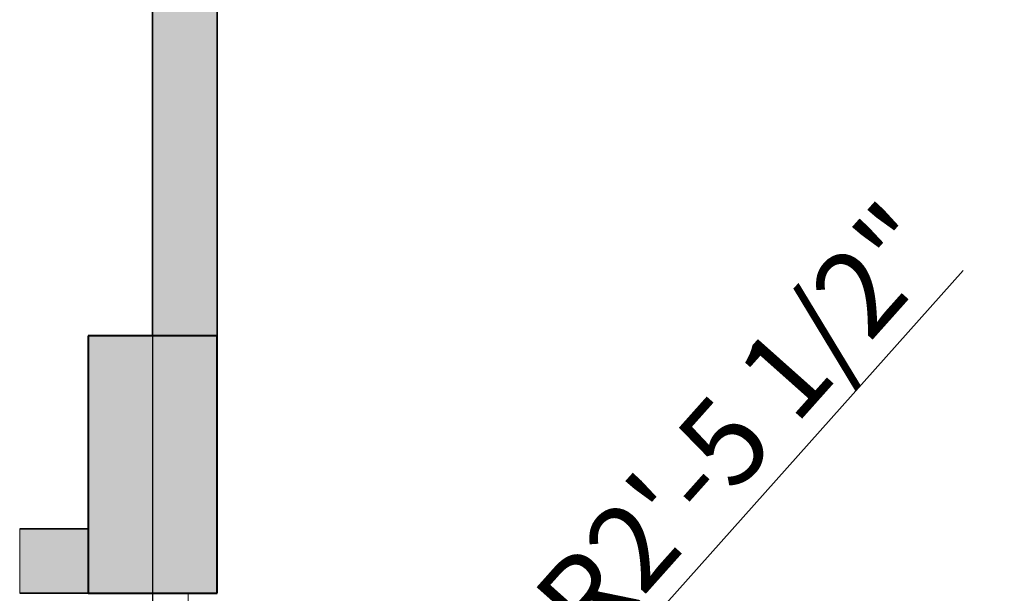
# Model space of a CAD drawing. Units: inches. Extents: x 2656 to 9931, y 1941 to 3068.
# Tile 14 of 46: x 2863 to 2932, y 2426 to 2466. Entities that reach past the tile are written whole.
import ezdxf

# ---------------------------------------------------------------- set-up
doc = ezdxf.new("R2010")
doc.units = ezdxf.units.IN
for name, color, linetype, lineweight in [('A-ANNO-DIMS', 2, 'Continuous', 18), ('A-COLS', 7, 'Continuous', 40), ('A-COLS-PATT', 146, 'Continuous', 13), ('A-DOOR', 3, 'Continuous', 18), ('A-WALL', 7, 'Continuous', 35), ('A-WALL-PATT', 251, 'Continuous', 13)]:
    doc.layers.add(name, color=color, linetype=linetype, lineweight=lineweight)
doc.styles.get("Standard").update_dxf_attribs({"font": 'arial.ttf'})
doc.dimstyles.new('ISO-25', dxfattribs={"dimtxt": 6, "dimasz": 2.5, "dimexe": 1.25, "dimexo": 0.625, "dimtad": 1, "dimdec": 0, "dimlunit": 3, "dimtxsty": 'Standard', "dimcen": 2.5, "dimadec": 0, "dimazin": 0, "dimtfac": 1, "dimtdec": 0, "dimtmove": 0, "dimatfit": 3, "dimfxl": 1, "dimarcsym": 0})

# ---------------------------------------------------------------- blocks, each defined once
blk = doc.blocks.new('DOOR-BEDROOM-HALL')
for p, q in [((-0.043, 0), (-0.043, 36)), ((2.43, 36), (2.43, 34)), ((38.43, 3), (2.43, 3)), ((2.43, 3), (2.43, 2)), ((38.43, 2), (38.43, 3)), ((2.43, 0), (2.43, 2)), ((2.43, 2), (38.43, 2))]:
    blk.add_line(p, q)
blk.add_arc((9.014, 5.243), 29.501, 353.68892, 102.89617)
blk = doc.blocks.new('*D102')
at = {"layer": 'A-ANNO-DIMS', "color": 0, "lineweight": -2, "transparency": 16777216}
for p, q in [((2998.157, 2604.975), (2998.157, 2009.273)), ((2872.157, 2564.712), (2872.157, 2009.273)), ((2874.657, 2010.523), (2995.657, 2010.523))]:
    blk.add_line(p, q, dxfattribs=at)
at = {"layer": 'A-ANNO-DIMS', "color": 0, "transparency": 16777216}
for points in [[(2874.657, 2010.939), (2874.657, 2010.106), (2872.157, 2010.523)], [(2995.657, 2010.939), (2995.657, 2010.106), (2998.157, 2010.523)]]:
    blk.add_solid(points, dxfattribs=at)
at = {"layer": 'Defpoints', "color": 0, "transparency": 16777216}
for p in [(2998.157, 2605.6), (2872.157, 2565.337), (2998.157, 2010.523)]:
    blk.add_point(p, dxfattribs=at)
at = {"layer": 'A-ANNO-DIMS', "color": 0, "transparency": 16777216, "insert": (2935.157, 2014.211), "char_height": 6, "attachment_point": 5}
blk.add_mtext('10\'-6"', dxfattribs=at)
blk = doc.blocks.new('*D185')
at = {"layer": 'A-ANNO-DIMS', "color": 0, "lineweight": -2, "transparency": 16777216}
for p, q in [((2928.735, 2448.665), (2902.506, 2419.234)), ((2881.214, 2395.343), (2900.842, 2417.367))]:
    blk.add_line(p, q, dxfattribs=at)
at = {"layer": 'A-ANNO-DIMS', "color": 0, "transparency": 16777216}
blk.add_solid([(2902.195, 2419.511), (2902.817, 2418.957), (2900.842, 2417.367)], dxfattribs=at)
at = {"layer": 'Defpoints', "color": 0, "transparency": 16777216}
for p in [(2900.842, 2417.367), (2881.214, 2395.343)]:
    blk.add_point(p, dxfattribs=at)
at = {"layer": 'A-ANNO-DIMS', "color": 0, "transparency": 16777216, "insert": (2913.669, 2437.362), "char_height": 6, "attachment_point": 5, "rotation": 48.29259}
blk.add_mtext('R2\'-5 1/2"', dxfattribs=at)

msp = doc.modelspace()

# ---------------------------------------------------------------- hatches: boundary and pattern name
at = {"layer": 'A-COLS-PATT'}
h = msp.add_hatch(color=256, dxfattribs=at)
h.dxf.hatch_style = 1
h.paths.add_polyline_path([(2752.157, 2623.6), (2743.157, 2623.6), (2743.157, 2605.6), (2752.157, 2605.6)])
h.paths.add_polyline_path([(2876.657, 2623.6), (2858.657, 2623.6), (2858.657, 2614.6), (2876.657, 2614.6)])
h.paths.add_polyline_path([(2998.157, 2623.6), (2989.157, 2623.6), (2989.157, 2614.6), (2989.157, 2605.6), (2998.157, 2605.6)])
h.paths.add_polyline_path([(2998.157, 2444.1), (2989.157, 2444.1), (2989.157, 2426.1), (2998.157, 2426.1)])
h.paths.add_polyline_path([(2876.657, 2444.1), (2867.657, 2444.1), (2867.657, 2426.1), (2876.657, 2426.1)])
h.paths.add_polyline_path([(2752.157, 2444.1), (2743.157, 2444.1), (2743.157, 2426.1), (2752.157, 2426.1)])
h.paths.add_polyline_path([(2752.157, 2300.1), (2743.157, 2300.1), (2743.157, 2282.1), (2752.157, 2282.1)])
h.paths.add_polyline_path([(2876.657, 2300.1), (2867.657, 2300.1), (2867.657, 2282.1), (2876.657, 2282.1)])
h.paths.add_polyline_path([(2998.157, 2300.1), (2989.157, 2300.1), (2989.157, 2282.1), (2998.157, 2282.1)])
h.paths.add_polyline_path([(2998.157, 2184.6), (2989.157, 2184.6), (2989.157, 2166.6), (2998.157, 2166.6)])
h.paths.add_polyline_path([(2876.657, 2175.6), (2858.657, 2175.6), (2858.657, 2166.6), (2876.657, 2166.6)])
h.paths.add_polyline_path([(2752.157, 2184.6), (2743.157, 2184.6), (2743.157, 2166.6), (2752.157, 2166.6)])
at = {"layer": 'A-WALL-PATT'}
h = msp.add_hatch(color=256, dxfattribs=at)
h.dxf.hatch_style = 1
h.paths.add_polyline_path([(2858.657, 2623.6), (2752.157, 2623.6), (2752.157, 2614.6), (2858.657, 2614.6)])
h.paths.add_polyline_path([(2893.087, 2623.6), (2876.657, 2623.6), (2876.657, 2614.6), (2893.087, 2614.6), (2893.087, 2619.1)])
h.paths.add_polyline_path([(2946.514, 2623.6), (2917.087, 2623.6), (2917.087, 2614.6), (2946.514, 2614.6), (2946.514, 2619.1)])
h.paths.add_polyline_path([(2989.157, 2623.6), (2970.514, 2623.6), (2970.514, 2614.6), (2989.157, 2614.6)])
h.paths.add_polyline_path([(2998.157, 2605.6), (2989.157, 2605.6), (2989.157, 2523.881), (2998.157, 2523.881)])
h.paths.add_polyline_path([(2935.157, 2614.6), (2930.657, 2614.6), (2930.657, 2554.6), (2876.657, 2554.6), (2876.657, 2565.337), (2872.157, 2565.337), (2872.157, 2444.1), (2876.657, 2444.1), (2876.657, 2550.1), (2946.472, 2550.1), (2946.472, 2554.6), (2935.157, 2554.6)])
h.paths.add_polyline_path([(2989.157, 2554.6), (2982.11, 2554.6), (2976.574, 2554.6), (2976.574, 2550.1), (2982.11, 2550.1), (2989.157, 2550.1)])
h.paths.add_polyline_path([(2876.657, 2614.6), (2872.157, 2614.6), (2872.157, 2595.003), (2876.657, 2595.003)], flags=0)
h.paths.add_polyline_path([(2752.157, 2605.6), (2743.157, 2605.6), (2743.157, 2544.033), (2752.157, 2544.033)])
h.paths.add_polyline_path([(2752.157, 2426.1), (2743.157, 2426.1), (2743.157, 2300.1), (2752.157, 2300.1)])
h.paths.add_polyline_path([(2821.134, 2430.6), (2752.157, 2430.6), (2752.157, 2426.1), (2821.134, 2426.1)])
h.paths.add_polyline_path([(2867.657, 2430.6), (2862.876, 2430.6), (2862.876, 2426.1), (2867.657, 2426.1)])
h.paths.add_polyline_path([(2752.157, 2484.033), (2747.657, 2484.033), (2743.157, 2484.033), (2743.157, 2444.1), (2752.157, 2444.1)])
h.paths.add_polyline_path([(2998.157, 2426.1), (2989.157, 2426.1), (2989.157, 2390.1), (2872.157, 2390.1), (2872.157, 2385.6), (2876.657, 2385.6), (2989.157, 2385.6), (2989.157, 2365.037), (2998.157, 2365.037)])
h.paths.add_polyline_path([(2998.157, 2463.881), (2993.657, 2463.881), (2989.157, 2463.881), (2989.157, 2444.1), (2998.157, 2444.1)])
h.paths.add_polyline_path([(2998.157, 2319.88), (2989.157, 2319.88), (2989.157, 2300.1), (2998.157, 2300.1)])
h.paths.add_polyline_path([(2998.157, 2282.1), (2989.157, 2282.1), (2989.157, 2253.6), (2982.058, 2253.6), (2982.058, 2249.1), (2989.157, 2249.1), (2998.157, 2249.1)])
h.paths.add_polyline_path([(2931.542, 2253.6), (2923.796, 2253.6), (2923.796, 2249.1), (2931.542, 2249.1)])
h.paths.add_polyline_path([(2876.657, 2282.1), (2872.157, 2282.1), (2872.157, 2184.6), (2872.157, 2175.6), (2876.657, 2175.6), (2876.657, 2249.1), (2888.323, 2249.1), (2888.323, 2251.35), (2888.323, 2253.6), (2876.657, 2253.6)])
h.paths.add_polyline_path([(2858.657, 2175.6), (2841.419, 2175.6), (2841.419, 2166.6), (2858.657, 2166.6)])
h.paths.add_polyline_path([(2785.058, 2171.1), (2785.058, 2175.6), (2752.157, 2175.6), (2752.157, 2166.6), (2785.058, 2166.6)])
h.paths.add_polyline_path([(2752.157, 2282.1), (2743.157, 2282.1), (2743.157, 2184.6), (2752.157, 2184.6)])
h.paths.add_polyline_path([(2809.769, 2300.1), (2752.157, 2300.1), (2752.157, 2295.6), (2809.769, 2295.6)])
h.paths.add_polyline_path([(2867.657, 2300.1), (2851.877, 2300.1), (2851.877, 2295.6), (2867.657, 2295.6)])

# ---------------------------------------------------------------- linework, layer by layer
at = {"layer": 'A-COLS'}
for p, q in [((2876.657, 2444.1), (2867.657, 2444.1)), ((2867.657, 2444.1), (2867.657, 2426.1)), ((2876.657, 2426.1), (2876.657, 2444.1)), ((2867.657, 2426.1), (2876.657, 2426.1))]:
    msp.add_line(p, q, dxfattribs=at)
at = {"layer": 'A-DOOR'}
msp.add_line((2862.876, 2430.6), (2862.876, 2426.1), dxfattribs=at)
at = {"layer": 'A-WALL'}
for p, q in [((2872.157, 2565.337), (2872.157, 2444.1)), ((2876.657, 2550.1), (2876.657, 2426.1)), ((2862.876, 2430.6), (2867.657, 2430.6)), ((2862.876, 2426.1), (2876.657, 2426.1))]:
    msp.add_line(p, q, dxfattribs=at)

# ---------------------------------------------------------------- block references
at = {"layer": 'A-DOOR'}
msp.add_blockref('DOOR-BEDROOM-HALL', (2872.2, 2390.1), dxfattribs=at)

# ---------------------------------------------------------------- dimensions: what is measured, and where the dimension line sits
at = {"layer": 'A-ANNO-DIMS'}
dim = msp.add_linear_dim(base=(2998.157, 2010.523), p1=(2872.157, 2565.337), p2=(2998.157, 2605.6), dimstyle='ISO-25', override={"dimdec": 1, "dimlfac": 1, "dimrnd": 0, "dimzin": 1, "dimdsep": 46, "dimlunit": 4, "dimfrac": 2}, dxfattribs=at)
dim.commit()
dim.dimension.update_dxf_attribs({"geometry": '*D102', "text_midpoint": (2935.157, 2014.211)})
dim = msp.add_radius_dim(center=(2881.214, 2395.343), mpoint=(2900.842, 2417.367), dimstyle='ISO-25', override={"dimdec": 1, "dimlfac": 1, "dimrnd": 0, "dimzin": 1, "dimdsep": 46, "dimlunit": 4, "dimfrac": 2}, dxfattribs=at)
dim.commit()
dim.dimension.update_dxf_attribs({"geometry": '*D185', "text_midpoint": (2913.669, 2437.362)})

doc.saveas('drawing.dxf')
